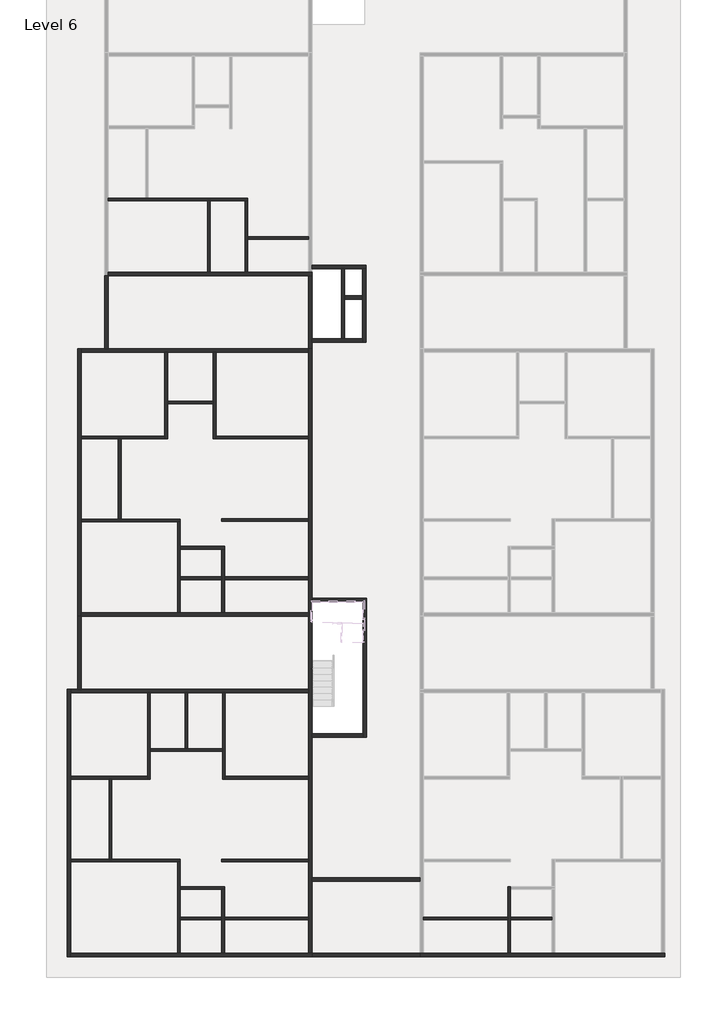
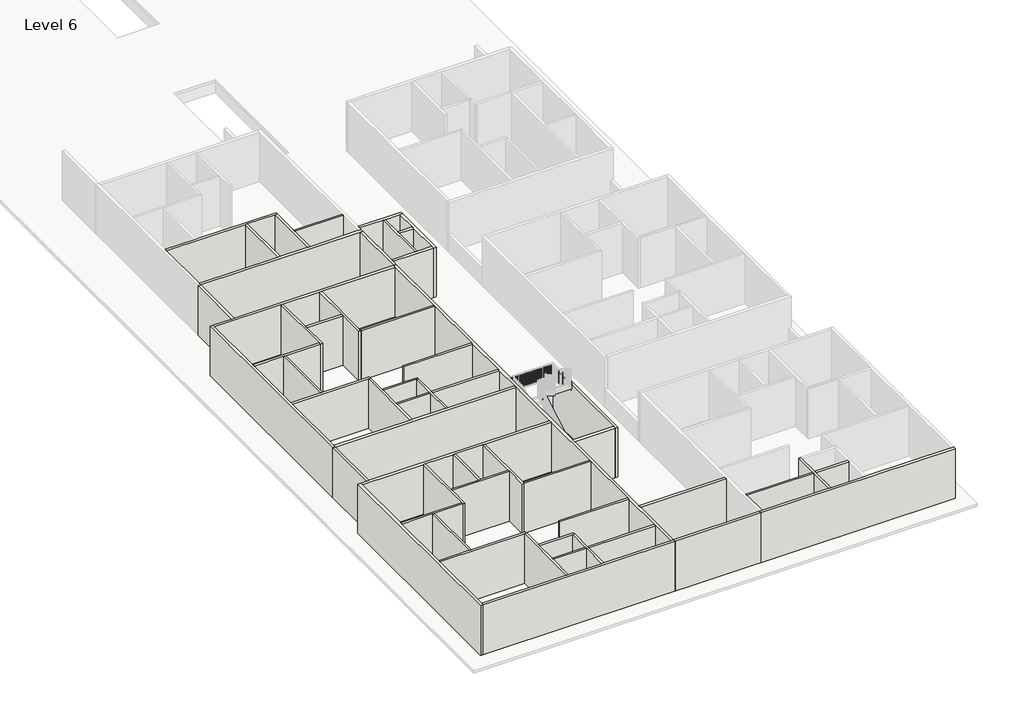
# One storey, part 1 of 8: 55 walls.
"""IFC4 building model written with IfcOpenShell, lengths in millimetres."""

from ifc_helpers import new_model, si_unit, frame, origin, place, context, project, spatial, polyline, outline, extrude, faceted_brep, element, save

model = new_model("IFC4")

# Units and contexts
model_context = context("Model", 3, world=origin())
ifc_project = project(units=[si_unit("LENGTHUNIT", "METRE", prefix="MILLI")], contexts=[model_context])

# Site, building, storey
site = spatial("IfcSite", under=ifc_project)
building = spatial("IfcBuilding", under=site)
storey = spatial("IfcBuildingStorey", under=building, Name="Level 6", Elevation=40474.6172466)

# Walls
placement = place(None, origin())
element("IfcWall", 1, ObjectType="4.5\"", at=placement, inside=storey, context=model_context, shape_type="Brep", body=[
    faceted_brep([(-12531.5544854, -1061.7344126, 40474.6172466), (-8188.1544854, -1061.7344126, 40474.6172466), (-8073.8544854, -1061.7344126, 40474.6172466), (-6549.8544854, -1061.7344126, 40474.6172466), (-6435.5544854, -1061.7344126, 40474.6172466), (-6435.5544854, -1061.7344126, 43522.6172466), (-6549.8544854, -1061.7344126, 43522.6172466), (-8073.8544854, -1061.7344126, 43522.6172466), (-8188.1544854, -1061.7344126, 43522.6172466), (-12531.5544854, -1061.7344126, 43522.6172466), (-12531.5544854, -947.4344126, 40474.6172466), (-12531.5544854, -947.4344126, 43522.6172466), (-10907.2415084, -947.4344126, 43522.6172466), (-10792.9415084, -947.4344126, 43522.6172466), (-6435.5544854, -947.4344126, 43522.6172466), (-6435.5544854, -947.4344126, 40474.6172466), (-10792.9415084, -947.4344126, 40474.6172466), (-10907.2415084, -947.4344126, 40474.6172466)], [[[0, 1, 2, 3, 4, 5, 6, 7, 8, 9]], [[10, 11, 12, 13, 14, 15, 16, 17]], [[4, 3, 2, 1, 0, 10, 17, 16, 15]], [[0, 9, 11, 10]], [[5, 4, 15, 14]], [[9, 8, 7, 6, 5, 14, 13, 12, 11]]]),
])
element("IfcWall", 2, ObjectType="4.5\"", at=placement, inside=storey, context=model_context, shape_type="Brep", body=[
    faceted_brep([(-6549.8544854, -1061.7344126, 40474.6172466), (-6549.8544854, -4185.9344126, 40474.6172466), (-6549.8544854, -4185.9344126, 43522.6172466), (-6549.8544854, -1061.7344126, 43522.6172466), (-6435.5544854, -1061.7344126, 40474.6172466), (-6435.5544854, -1061.7344126, 43522.6172466), (-6435.5544854, -2623.8344126, 43522.6172466), (-6435.5544854, -2738.1344126, 43522.6172466), (-6435.5544854, -4185.9344126, 43522.6172466), (-6435.5544854, -4185.9344126, 40474.6172466), (-6435.5544854, -2738.1344126, 40474.6172466), (-6435.5544854, -2623.8344126, 40474.6172466)], [[[0, 1, 2, 3]], [[4, 5, 6, 7, 8, 9, 10, 11]], [[1, 0, 4, 11, 10, 9]], [[0, 3, 5, 4]], [[2, 1, 9, 8]], [[3, 2, 8, 7, 6, 5]]]),
])
element("IfcWall", 3, ObjectType="4.5\"", at=placement, inside=storey, context=model_context, shape_type="SweptSolid", body=[
    extrude(outline(polyline([(-8188.1544854, -4185.9344126), (-8188.1544854, -1061.7344126), (-8073.8544854, -1061.7344126), (-8073.8544854, -4185.9344126), (-8188.1544854, -4185.9344126)])), frame((0.0, 0.0, 40474.6172466), z_axis=(0.0, 0.0, 1.0), x_axis=(1.0, 0.0, 0.0)), (0.0, 0.0, 1.0), 3048.0),
])
element("IfcWall", 4, ObjectType="4.5\"", at=placement, inside=storey, context=model_context, shape_type="SweptSolid", body=[
    extrude(outline(polyline([(-6435.5544854, -2623.8344126), (-3769.8415084, -2623.8344126), (-3769.8415084, -2738.1344126), (-6435.5544854, -2738.1344126), (-6435.5544854, -2623.8344126)])), frame((0.0, 0.0, 40474.6172466), z_axis=(0.0, 0.0, 1.0), x_axis=(1.0, 0.0, 0.0)), (0.0, 0.0, 1.0), 3048.0),
])
element("IfcWall", 5, ObjectType="4.5\"", at=placement, inside=storey, context=model_context, shape_type="Brep", body=[
    faceted_brep([(-10061.4044854, -7691.1344126, 40474.6172466), (-10061.4044854, -11348.7344126, 40474.6172466), (-10061.4044854, -11463.0344126, 40474.6172466), (-10061.4044854, -11463.0344126, 43522.6172466), (-10061.4044854, -11348.7344126, 43522.6172466), (-10061.4044854, -7691.1344126, 43522.6172466), (-9947.1044854, -7691.1344126, 40474.6172466), (-9947.1044854, -7691.1344126, 43522.6172466), (-9947.1044854, -9824.7344126, 43522.6172466), (-9947.1044854, -9939.0344126, 43522.6172466), (-9947.1044854, -11463.0344126, 43522.6172466), (-9947.1044854, -11463.0344126, 40474.6172466), (-9947.1044854, -9939.0344126, 40474.6172466), (-9947.1044854, -9824.7344126, 40474.6172466)], [[[0, 1, 2, 3, 4, 5]], [[6, 7, 8, 9, 10, 11, 12, 13]], [[2, 1, 0, 6, 13, 12, 11]], [[0, 5, 7, 6]], [[3, 2, 11, 10]], [[5, 4, 3, 10, 9, 8, 7]]]),
])
element("IfcWall", 6, ObjectType="4.5\"", at=placement, inside=storey, context=model_context, shape_type="Brep", body=[
    faceted_brep([(-10061.4044854, -11348.7344126, 40474.6172466), (-13719.0044854, -11348.7344126, 40474.6172466), (-13719.0044854, -11348.7344126, 43522.6172466), (-10061.4044854, -11348.7344126, 43522.6172466), (-10061.4044854, -11463.0344126, 40474.6172466), (-10061.4044854, -11463.0344126, 43522.6172466), (-11980.3915084, -11463.0344126, 43522.6172466), (-12094.6915084, -11463.0344126, 43522.6172466), (-13719.0044854, -11463.0344126, 43522.6172466), (-13719.0044854, -11463.0344126, 40474.6172466), (-12094.6915084, -11463.0344126, 40474.6172466), (-11980.3915084, -11463.0344126, 40474.6172466)], [[[0, 1, 2, 3]], [[4, 5, 6, 7, 8, 9, 10, 11]], [[1, 0, 4, 11, 10, 9]], [[0, 3, 5, 4]], [[2, 1, 9, 8]], [[3, 2, 8, 7, 6, 5]]]),
])
element("IfcWall", 7, ObjectType="4.5\"", at=placement, inside=storey, context=model_context, shape_type="SweptSolid", body=[
    extrude(outline(polyline([(-12094.6915084, -14968.2344126), (-12094.6915084, -11463.0344126), (-11980.3915084, -11463.0344126), (-11980.3915084, -14968.2344126), (-12094.6915084, -14968.2344126)])), frame((0.0, 0.0, 40474.6172466), z_axis=(0.0, 0.0, 1.0), x_axis=(1.0, 0.0, 0.0)), (0.0, 0.0, 1.0), 3048.0),
])
element("IfcWall", 8, ObjectType="4.5\"", at=placement, inside=storey, context=model_context, shape_type="Brep", body=[
    faceted_brep([(-13719.0044854, -15095.2344126, 40474.6172466), (-9510.2415084, -15095.2344126, 40474.6172466), (-9395.9415084, -15095.2344126, 40474.6172466), (-9395.9415084, -15095.2344126, 43522.6172466), (-9510.2415084, -15095.2344126, 43522.6172466), (-13719.0044854, -15095.2344126, 43522.6172466), (-13719.0044854, -14980.9344126, 40474.6172466), (-13719.0044854, -14980.9344126, 43522.6172466), (-9395.9415084, -14980.9344126, 43522.6172466), (-9395.9415084, -14980.9344126, 40474.6172466)], [[[0, 1, 2, 3, 4, 5]], [[6, 7, 8, 9]], [[2, 1, 0, 6, 9]], [[0, 5, 7, 6]], [[3, 2, 9, 8]], [[5, 4, 3, 8, 7]]]),
])
element("IfcWall", 9, ObjectType="4.5\"", at=placement, inside=storey, context=model_context, shape_type="Brep", body=[
    faceted_brep([(-9510.2415084, -15095.2344126, 40474.6172466), (-9510.2415084, -19070.3344126, 40474.6172466), (-9510.2415084, -19070.3344126, 43522.6172466), (-9510.2415084, -15095.2344126, 43522.6172466), (-9395.9415084, -15095.2344126, 40474.6172466), (-9395.9415084, -15095.2344126, 43522.6172466), (-9395.9415084, -16174.7344126, 43522.6172466), (-9395.9415084, -16289.0344126, 43522.6172466), (-9395.9415084, -17508.2344126, 43522.6172466), (-9395.9415084, -17622.5344126, 43522.6172466), (-9395.9415084, -19070.3344126, 43522.6172466), (-9395.9415084, -19070.3344126, 40474.6172466), (-9395.9415084, -17622.5344126, 40474.6172466), (-9395.9415084, -17508.2344126, 40474.6172466), (-9395.9415084, -16289.0344126, 40474.6172466), (-9395.9415084, -16174.7344126, 40474.6172466)], [[[0, 1, 2, 3]], [[4, 5, 6, 7, 8, 9, 10, 11, 12, 13, 14, 15]], [[1, 0, 4, 15, 14, 13, 12, 11]], [[0, 3, 5, 4]], [[2, 1, 11, 10]], [[3, 2, 10, 9, 8, 7, 6, 5]]]),
])
element("IfcWall", 10, ObjectType="4.5\"", at=placement, inside=storey, context=model_context, shape_type="Brep", body=[
    faceted_brep([(-9395.9415084, -16289.0344126, 40474.6172466), (-7567.1415084, -16289.0344126, 40474.6172466), (-7452.8415084, -16289.0344126, 40474.6172466), (-7452.8415084, -16289.0344126, 43522.6172466), (-7567.1415084, -16289.0344126, 43522.6172466), (-9395.9415084, -16289.0344126, 43522.6172466), (-9395.9415084, -16174.7344126, 40474.6172466), (-9395.9415084, -16174.7344126, 43522.6172466), (-7452.8415084, -16174.7344126, 43522.6172466), (-7452.8415084, -16174.7344126, 40474.6172466)], [[[0, 1, 2, 3, 4, 5]], [[6, 7, 8, 9]], [[2, 1, 0, 6, 9]], [[0, 5, 7, 6]], [[3, 2, 9, 8]], [[5, 4, 3, 8, 7]]]),
])
element("IfcWall", 11, ObjectType="4.5\"", at=placement, inside=storey, context=model_context, shape_type="Brep", body=[
    faceted_brep([(-7567.1415084, -16289.0344126, 40474.6172466), (-7567.1415084, -17508.2344126, 40474.6172466), (-7567.1415084, -17622.5344126, 40474.6172466), (-7567.1415084, -19070.3344126, 40474.6172466), (-7567.1415084, -19070.3344126, 43522.6172466), (-7567.1415084, -17622.5344126, 43522.6172466), (-7567.1415084, -17508.2344126, 43522.6172466), (-7567.1415084, -16289.0344126, 43522.6172466), (-7452.8415084, -16289.0344126, 40474.6172466), (-7452.8415084, -16289.0344126, 43522.6172466), (-7452.8415084, -17508.2344126, 43522.6172466), (-7452.8415084, -17622.5344126, 43522.6172466), (-7452.8415084, -19070.3344126, 43522.6172466), (-7452.8415084, -19070.3344126, 40474.6172466), (-7452.8415084, -17622.5344126, 40474.6172466), (-7452.8415084, -17508.2344126, 40474.6172466)], [[[0, 1, 2, 3, 4, 5, 6, 7]], [[8, 9, 10, 11, 12, 13, 14, 15]], [[3, 2, 1, 0, 8, 15, 14, 13]], [[0, 7, 9, 8]], [[4, 3, 13, 12]], [[7, 6, 5, 4, 12, 11, 10, 9]]]),
])
element("IfcWall", 12, ObjectType="4.5\"", at=placement, inside=storey, context=model_context, shape_type="SweptSolid", body=[
    extrude(outline(polyline([(-7567.1415084, -17622.5344126), (-9395.9415084, -17622.5344126), (-9395.9415084, -17508.2344126), (-7567.1415084, -17508.2344126), (-7567.1415084, -17622.5344126)])), frame((0.0, 0.0, 40474.6172466), z_axis=(0.0, 0.0, 1.0), x_axis=(1.0, 0.0, 0.0)), (0.0, 0.0, 1.0), 3048.0),
])
element("IfcWall", 13, ObjectType="4.5\"", at=placement, inside=storey, context=model_context, shape_type="SweptSolid", body=[
    extrude(outline(polyline([(-3769.8415084, -17622.5344126), (-7452.8415084, -17622.5344126), (-7452.8415084, -17508.2344126), (-3769.8415084, -17508.2344126), (-3769.8415084, -17622.5344126)])), frame((0.0, 0.0, 40474.6172466), z_axis=(0.0, 0.0, 1.0), x_axis=(1.0, 0.0, 0.0)), (0.0, 0.0, 1.0), 3048.0),
])
element("IfcWall", 14, ObjectType="4.5\"", at=placement, inside=storey, context=model_context, shape_type="SweptSolid", body=[
    extrude(outline(polyline([(-7567.1415084, -14968.2344126), (-3769.8415084, -14968.2344126), (-3769.8415084, -15082.5344126), (-7567.1415084, -15082.5344126), (-7567.1415084, -14968.2344126)])), frame((0.0, 0.0, 40474.6172466), z_axis=(0.0, 0.0, 1.0), x_axis=(1.0, 0.0, 0.0)), (0.0, 0.0, 1.0), 3048.0),
])
element("IfcWall", 15, ObjectType="4.5\"", at=placement, inside=storey, context=model_context, shape_type="SweptSolid", body=[
    extrude(outline(polyline([(-7940.5044854, -9939.0344126), (-9947.1044854, -9939.0344126), (-9947.1044854, -9824.7344126), (-7940.5044854, -9824.7344126), (-7940.5044854, -9939.0344126)])), frame((0.0, 0.0, 40474.6172466), z_axis=(0.0, 0.0, 1.0), x_axis=(1.0, 0.0, 0.0)), (0.0, 0.0, 1.0), 3048.0),
])
element("IfcWall", 16, ObjectType="4.5\"", at=placement, inside=storey, context=model_context, shape_type="Brep", body=[
    faceted_brep([(-7940.5044854, -7691.1344126, 40474.6172466), (-7940.5044854, -9824.7344126, 40474.6172466), (-7940.5044854, -9939.0344126, 40474.6172466), (-7940.5044854, -11463.0344126, 40474.6172466), (-7940.5044854, -11463.0344126, 43522.6172466), (-7940.5044854, -9939.0344126, 43522.6172466), (-7940.5044854, -9824.7344126, 43522.6172466), (-7940.5044854, -7691.1344126, 43522.6172466), (-7826.2044854, -7691.1344126, 40474.6172466), (-7826.2044854, -7691.1344126, 43522.6172466), (-7826.2044854, -11348.7344126, 43522.6172466), (-7826.2044854, -11463.0344126, 43522.6172466), (-7826.2044854, -11463.0344126, 40474.6172466), (-7826.2044854, -11348.7344126, 40474.6172466)], [[[0, 1, 2, 3, 4, 5, 6, 7]], [[8, 9, 10, 11, 12, 13]], [[3, 2, 1, 0, 8, 13, 12]], [[0, 7, 9, 8]], [[4, 3, 12, 11]], [[7, 6, 5, 4, 11, 10, 9]]]),
])
element("IfcWall", 17, ObjectType="4.5\"", at=placement, inside=storey, context=model_context, shape_type="SweptSolid", body=[
    extrude(outline(polyline([(-3769.8415084, -11463.0344126), (-7826.2044854, -11463.0344126), (-7826.2044854, -11348.7344126), (-3769.8415084, -11348.7344126), (-3769.8415084, -11463.0344126)])), frame((0.0, 0.0, 40474.6172466), z_axis=(0.0, 0.0, 1.0), x_axis=(1.0, 0.0, 0.0)), (0.0, 0.0, 1.0), 3048.0),
])
element("IfcWall", 18, ObjectType="4.5\"", at=placement, inside=storey, context=model_context, shape_type="Brep", body=[
    faceted_brep([(-10818.3415084, -22575.5344126, 40474.6172466), (-10818.3415084, -26233.1344126, 40474.6172466), (-10818.3415084, -26347.4344126, 40474.6172466), (-10818.3415084, -26347.4344126, 43522.6172466), (-10818.3415084, -26233.1344126, 43522.6172466), (-10818.3415084, -22575.5344126, 43522.6172466), (-10704.0415084, -22575.5344126, 40474.6172466), (-10704.0415084, -22575.5344126, 43522.6172466), (-10704.0415084, -25013.9344126, 43522.6172466), (-10704.0415084, -25128.2344126, 43522.6172466), (-10704.0415084, -26347.4344126, 43522.6172466), (-10704.0415084, -26347.4344126, 40474.6172466), (-10704.0415084, -25128.2344126, 40474.6172466), (-10704.0415084, -25013.9344126, 40474.6172466)], [[[0, 1, 2, 3, 4, 5]], [[6, 7, 8, 9, 10, 11, 12, 13]], [[2, 1, 0, 6, 13, 12, 11]], [[0, 5, 7, 6]], [[3, 2, 11, 10]], [[5, 4, 3, 10, 9, 8, 7]]]),
])
element("IfcWall", 19, ObjectType="4.5\"", at=placement, inside=storey, context=model_context, shape_type="Brep", body=[
    faceted_brep([(-10818.3415084, -26233.1344126, 40474.6172466), (-14171.1415084, -26233.1344126, 40474.6172466), (-14171.1415084, -26233.1344126, 43522.6172466), (-10818.3415084, -26233.1344126, 43522.6172466), (-10818.3415084, -26347.4344126, 40474.6172466), (-10818.3415084, -26347.4344126, 43522.6172466), (-12380.4415084, -26347.4344126, 43522.6172466), (-12494.7415084, -26347.4344126, 43522.6172466), (-14171.1415084, -26347.4344126, 43522.6172466), (-14171.1415084, -26347.4344126, 40474.6172466), (-12494.7415084, -26347.4344126, 40474.6172466), (-12380.4415084, -26347.4344126, 40474.6172466)], [[[0, 1, 2, 3]], [[4, 5, 6, 7, 8, 9, 10, 11]], [[1, 0, 4, 11, 10, 9]], [[0, 3, 5, 4]], [[2, 1, 9, 8]], [[3, 2, 8, 7, 6, 5]]]),
])
element("IfcWall", 20, ObjectType="4.5\"", at=placement, inside=storey, context=model_context, shape_type="SweptSolid", body=[
    extrude(outline(polyline([(-9180.0415084, -25013.9344126), (-9180.0415084, -22575.5344126), (-9065.7415084, -22575.5344126), (-9065.7415084, -25013.9344126), (-9180.0415084, -25013.9344126)])), frame((0.0, 0.0, 40474.6172466), z_axis=(0.0, 0.0, 1.0), x_axis=(1.0, 0.0, 0.0)), (0.0, 0.0, 1.0), 3048.0),
])
element("IfcWall", 21, ObjectType="4.5\"", at=placement, inside=storey, context=model_context, shape_type="Brep", body=[
    faceted_brep([(-10704.0415084, -25128.2344126, 40474.6172466), (-7541.7415084, -25128.2344126, 40474.6172466), (-7541.7415084, -25128.2344126, 43522.6172466), (-10704.0415084, -25128.2344126, 43522.6172466), (-10704.0415084, -25013.9344126, 40474.6172466), (-10704.0415084, -25013.9344126, 43522.6172466), (-9180.0415084, -25013.9344126, 43522.6172466), (-9065.7415084, -25013.9344126, 43522.6172466), (-7541.7415084, -25013.9344126, 43522.6172466), (-7541.7415084, -25013.9344126, 40474.6172466), (-9065.7415084, -25013.9344126, 40474.6172466), (-9180.0415084, -25013.9344126, 40474.6172466)], [[[0, 1, 2, 3]], [[4, 5, 6, 7, 8, 9, 10, 11]], [[1, 0, 4, 11, 10, 9]], [[0, 3, 5, 4]], [[2, 1, 9, 8]], [[3, 2, 8, 7, 6, 5]]]),
])
element("IfcWall", 22, ObjectType="4.5\"", at=placement, inside=storey, context=model_context, shape_type="Brep", body=[
    faceted_brep([(-7541.7415084, -22575.5344126, 40474.6172466), (-7541.7415084, -25013.9344126, 40474.6172466), (-7541.7415084, -25128.2344126, 40474.6172466), (-7541.7415084, -26347.4344126, 40474.6172466), (-7541.7415084, -26347.4344126, 43522.6172466), (-7541.7415084, -25128.2344126, 43522.6172466), (-7541.7415084, -25013.9344126, 43522.6172466), (-7541.7415084, -22575.5344126, 43522.6172466), (-7427.4415084, -22575.5344126, 40474.6172466), (-7427.4415084, -22575.5344126, 43522.6172466), (-7427.4415084, -26233.1344126, 43522.6172466), (-7427.4415084, -26347.4344126, 43522.6172466), (-7427.4415084, -26347.4344126, 40474.6172466), (-7427.4415084, -26233.1344126, 40474.6172466)], [[[0, 1, 2, 3, 4, 5, 6, 7]], [[8, 9, 10, 11, 12, 13]], [[3, 2, 1, 0, 8, 13, 12]], [[0, 7, 9, 8]], [[4, 3, 12, 11]], [[7, 6, 5, 4, 11, 10, 9]]]),
])
element("IfcWall", 23, ObjectType="4.5\"", at=placement, inside=storey, context=model_context, shape_type="SweptSolid", body=[
    extrude(outline(polyline([(-3769.8415084, -26347.4344126), (-7427.4415084, -26347.4344126), (-7427.4415084, -26233.1344126), (-3769.8415084, -26233.1344126), (-3769.8415084, -26347.4344126)])), frame((0.0, 0.0, 40474.6172466), z_axis=(0.0, 0.0, 1.0), x_axis=(1.0, 0.0, 0.0)), (0.0, 0.0, 1.0), 3048.0),
])
element("IfcWall", 24, ObjectType="4.5\"", at=placement, inside=storey, context=model_context, shape_type="SweptSolid", body=[
    extrude(outline(polyline([(-12494.7415084, -29852.6344126), (-12494.7415084, -26347.4344126), (-12380.4415084, -26347.4344126), (-12380.4415084, -29852.6344126), (-12494.7415084, -29852.6344126)])), frame((0.0, 0.0, 40474.6172466), z_axis=(0.0, 0.0, 1.0), x_axis=(1.0, 0.0, 0.0)), (0.0, 0.0, 1.0), 3048.0),
])
element("IfcWall", 25, ObjectType="4.5\"", at=placement, inside=storey, context=model_context, shape_type="Brep", body=[
    faceted_brep([(-14171.1415084, -29966.9344126, 40474.6172466), (-9510.2415084, -29966.9344126, 40474.6172466), (-9395.9415084, -29966.9344126, 40474.6172466), (-9395.9415084, -29966.9344126, 43522.6172466), (-9510.2415084, -29966.9344126, 43522.6172466), (-14171.1415084, -29966.9344126, 43522.6172466), (-14171.1415084, -29852.6344126, 40474.6172466), (-14171.1415084, -29852.6344126, 43522.6172466), (-12494.7415084, -29852.6344126, 43522.6172466), (-12380.4415084, -29852.6344126, 43522.6172466), (-9395.9415084, -29852.6344126, 43522.6172466), (-9395.9415084, -29852.6344126, 40474.6172466), (-12380.4415084, -29852.6344126, 40474.6172466), (-12494.7415084, -29852.6344126, 40474.6172466)], [[[0, 1, 2, 3, 4, 5]], [[6, 7, 8, 9, 10, 11, 12, 13]], [[2, 1, 0, 6, 13, 12, 11]], [[0, 5, 7, 6]], [[3, 2, 11, 10]], [[5, 4, 3, 10, 9, 8, 7]]]),
])
element("IfcWall", 26, ObjectType="4.5\"", at=placement, inside=storey, context=model_context, shape_type="Brep", body=[
    faceted_brep([(-9510.2415084, -29966.9344126, 40474.6172466), (-9510.2415084, -33954.7344126, 40474.6172466), (-9510.2415084, -33954.7344126, 43522.6172466), (-9510.2415084, -29966.9344126, 43522.6172466), (-9395.9415084, -29966.9344126, 40474.6172466), (-9395.9415084, -29966.9344126, 43522.6172466), (-9395.9415084, -31059.1344126, 43522.6172466), (-9395.9415084, -31173.4344126, 43522.6172466), (-9395.9415084, -32392.6344126, 43522.6172466), (-9395.9415084, -32506.9344126, 43522.6172466), (-9395.9415084, -33954.7344126, 43522.6172466), (-9395.9415084, -33954.7344126, 40474.6172466), (-9395.9415084, -32506.9344126, 40474.6172466), (-9395.9415084, -32392.6344126, 40474.6172466), (-9395.9415084, -31173.4344126, 40474.6172466), (-9395.9415084, -31059.1344126, 40474.6172466)], [[[0, 1, 2, 3]], [[4, 5, 6, 7, 8, 9, 10, 11, 12, 13, 14, 15]], [[1, 0, 4, 15, 14, 13, 12, 11]], [[0, 3, 5, 4]], [[2, 1, 11, 10]], [[3, 2, 10, 9, 8, 7, 6, 5]]]),
])
element("IfcWall", 27, ObjectType="4.5\"", at=placement, inside=storey, context=model_context, shape_type="Brep", body=[
    faceted_brep([(-9395.9415084, -31173.4344126, 40474.6172466), (-7567.1415084, -31173.4344126, 40474.6172466), (-7452.8415084, -31173.4344126, 40474.6172466), (-7452.8415084, -31173.4344126, 43522.6172466), (-7567.1415084, -31173.4344126, 43522.6172466), (-9395.9415084, -31173.4344126, 43522.6172466), (-9395.9415084, -31059.1344126, 40474.6172466), (-9395.9415084, -31059.1344126, 43522.6172466), (-7452.8415084, -31059.1344126, 43522.6172466), (-7452.8415084, -31059.1344126, 40474.6172466)], [[[0, 1, 2, 3, 4, 5]], [[6, 7, 8, 9]], [[2, 1, 0, 6, 9]], [[0, 5, 7, 6]], [[3, 2, 9, 8]], [[5, 4, 3, 8, 7]]]),
])
element("IfcWall", 28, ObjectType="4.5\"", at=placement, inside=storey, context=model_context, shape_type="Brep", body=[
    faceted_brep([(-7567.1415084, -31173.4344126, 40474.6172466), (-7567.1415084, -32392.6344126, 40474.6172466), (-7567.1415084, -32506.9344126, 40474.6172466), (-7567.1415084, -33954.7344126, 40474.6172466), (-7567.1415084, -33954.7344126, 43522.6172466), (-7567.1415084, -32506.9344126, 43522.6172466), (-7567.1415084, -32392.6344126, 43522.6172466), (-7567.1415084, -31173.4344126, 43522.6172466), (-7452.8415084, -31173.4344126, 40474.6172466), (-7452.8415084, -31173.4344126, 43522.6172466), (-7452.8415084, -32392.6344126, 43522.6172466), (-7452.8415084, -32506.9344126, 43522.6172466), (-7452.8415084, -33954.7344126, 43522.6172466), (-7452.8415084, -33954.7344126, 40474.6172466), (-7452.8415084, -32506.9344126, 40474.6172466), (-7452.8415084, -32392.6344126, 40474.6172466)], [[[0, 1, 2, 3, 4, 5, 6, 7]], [[8, 9, 10, 11, 12, 13, 14, 15]], [[3, 2, 1, 0, 8, 15, 14, 13]], [[0, 7, 9, 8]], [[4, 3, 13, 12]], [[7, 6, 5, 4, 12, 11, 10, 9]]]),
])
element("IfcWall", 29, ObjectType="4.5\"", at=placement, inside=storey, context=model_context, shape_type="SweptSolid", body=[
    extrude(outline(polyline([(-3769.8415084, -32392.6344126), (-3769.8415084, -32506.9344126), (-7452.8415084, -32506.9344126), (-7452.8415084, -32392.6344126), (-3769.8415084, -32392.6344126)])), frame((0.0, 0.0, 40474.6172466), z_axis=(0.0, 0.0, 1.0), x_axis=(1.0, 0.0, 0.0)), (0.0, 0.0, 1.0), 3048.0),
    extrude(outline(polyline([(-9395.9415084, -32506.9344126), (-9395.9415084, -32392.6344126), (-7567.1415084, -32392.6344126), (-7567.1415084, -32506.9344126), (-9395.9415084, -32506.9344126)])), frame((0.0, 0.0, 40474.6172466), z_axis=(0.0, 0.0, 1.0), x_axis=(1.0, 0.0, 0.0)), (0.0, 0.0, 1.0), 3048.0),
])
element("IfcWall", 30, ObjectType="4.5\"", at=placement, inside=storey, context=model_context, shape_type="SweptSolid", body=[
    extrude(outline(polyline([(-7567.1415084, -29852.6344126), (-3769.8415084, -29852.6344126), (-3769.8415084, -29966.9344126), (-7567.1415084, -29966.9344126), (-7567.1415084, -29852.6344126)])), frame((0.0, 0.0, 40474.6172466), z_axis=(0.0, 0.0, 1.0), x_axis=(1.0, 0.0, 0.0)), (0.0, 0.0, 1.0), 3048.0),
])
element("IfcWall", 31, ObjectType="4.5\"", at=placement, inside=storey, context=model_context, shape_type="SweptSolid", body=[
    extrude(outline(polyline([(4942.3584916, -32506.9344126), (1259.3584916, -32506.9344126), (1259.3584916, -32392.6344126), (4942.3584916, -32392.6344126), (4942.3584916, -32506.9344126)])), frame((0.0, 0.0, 40474.6172466), z_axis=(0.0, 0.0, 1.0), x_axis=(1.0, 0.0, 0.0)), (0.0, 0.0, 1.0), 3048.0),
])
element("IfcWall", 32, ObjectType="4.5\"", at=placement, inside=storey, context=model_context, shape_type="Brep", body=[
    faceted_brep([(4942.3584916, -31059.1344126, 40474.6172466), (4942.3584916, -32392.6344126, 40474.6172466), (4942.3584916, -32506.9344126, 40474.6172466), (4942.3584916, -33954.7344126, 40474.6172466), (4942.3584916, -33954.7344126, 43522.6172466), (4942.3584916, -32506.9344126, 43522.6172466), (4942.3584916, -32392.6344126, 43522.6172466), (4942.3584916, -31059.1344126, 43522.6172466), (5056.6584916, -31059.1344126, 40474.6172466), (5056.6584916, -31059.1344126, 43522.6172466), (5056.6584916, -31173.4344126, 43522.6172466), (5056.6584916, -32392.6344126, 43522.6172466), (5056.6584916, -32506.9344126, 43522.6172466), (5056.6584916, -33954.7344126, 43522.6172466), (5056.6584916, -33954.7344126, 40474.6172466), (5056.6584916, -32506.9344126, 40474.6172466), (5056.6584916, -32392.6344126, 40474.6172466), (5056.6584916, -31173.4344126, 40474.6172466)], [[[0, 1, 2, 3, 4, 5, 6, 7]], [[8, 9, 10, 11, 12, 13, 14, 15, 16, 17]], [[3, 2, 1, 0, 8, 17, 16, 15, 14]], [[4, 3, 14, 13]], [[0, 7, 9, 8]], [[7, 6, 5, 4, 13, 12, 11, 10, 9]]]),
])
element("IfcWall", 33, ObjectType="4.5\"", at=placement, inside=storey, context=model_context, shape_type="SweptSolid", body=[
    extrude(outline(polyline([(6885.4584916, -32506.9344126), (5056.6584916, -32506.9344126), (5056.6584916, -32392.6344126), (6885.4584916, -32392.6344126), (6885.4584916, -32506.9344126)])), frame((0.0, 0.0, 40474.6172466), z_axis=(0.0, 0.0, 1.0), x_axis=(1.0, 0.0, 0.0)), (0.0, 0.0, 1.0), 3048.0),
])
element("IfcWall", 34, ObjectType="4.5\"", at=placement, inside=storey, context=model_context, shape_type="Brep", body=[
    faceted_brep([(-2207.6738684, -7082.6751812, 40474.6172466), (-2207.6738684, -5366.3479894, 40474.6172466), (-2207.6738684, -5213.9479894, 40474.6172466), (-2207.6738684, -4034.6751812, 40474.6172466), (-2207.6738684, -4034.6751812, 43522.6172466), (-2207.6738684, -5213.9479894, 43522.6172466), (-2207.6738684, -5366.3479894, 43522.6172466), (-2207.6738684, -7082.6751812, 43522.6172466), (-2321.9738684, -7082.6751812, 40474.6172466), (-2321.9738684, -7082.6751812, 43522.6172466), (-2321.9738684, -4034.6751812, 43522.6172466), (-2321.9738684, -4034.6751812, 40474.6172466)], [[[0, 1, 2, 3, 4, 5, 6, 7]], [[8, 9, 10, 11]], [[3, 2, 1, 0, 8, 11]], [[7, 6, 5, 4, 10, 9]], [[4, 3, 11, 10]], [[0, 7, 9, 8]]]),
])
element("IfcWall", 35, ObjectType="6\"", at=placement, inside=storey, context=model_context, shape_type="Brep", body=[
    faceted_brep([(-12531.5544854, -4338.3344126, 40474.6172466), (-3769.8415084, -4338.3344126, 40474.6172466), (-3617.4415084, -4338.3344126, 40474.6172466), (-3617.4415084, -4338.3344126, 43522.6172466), (-3769.8415084, -4338.3344126, 43522.6172466), (-12531.5544854, -4338.3344126, 43522.6172466), (-12531.5544854, -4185.9344126, 40474.6172466), (-12531.5544854, -4185.9344126, 43522.6172466), (-8188.1544854, -4185.9344126, 43522.6172466), (-8073.8544854, -4185.9344126, 43522.6172466), (-6549.8544854, -4185.9344126, 43522.6172466), (-6435.5544854, -4185.9344126, 43522.6172466), (-3769.8415084, -4185.9344126, 43522.6172466), (-3617.4415084, -4185.9344126, 43522.6172466), (-3617.4415084, -4185.9344126, 40474.6172466), (-3769.8415084, -4185.9344126, 40474.6172466), (-6435.5544854, -4185.9344126, 40474.6172466), (-6549.8544854, -4185.9344126, 40474.6172466), (-8073.8544854, -4185.9344126, 40474.6172466), (-8188.1544854, -4185.9344126, 40474.6172466)], [[[0, 1, 2, 3, 4, 5]], [[6, 7, 8, 9, 10, 11, 12, 13, 14, 15, 16, 17, 18, 19]], [[2, 1, 0, 6, 19, 18, 17, 16, 15, 14]], [[0, 5, 7, 6]], [[3, 2, 14, 13]], [[5, 4, 3, 13, 12, 11, 10, 9, 8, 7]]]),
])
element("IfcWall", 36, ObjectType="6\"", at=placement, inside=storey, context=model_context, shape_type="Brep", body=[
    faceted_brep([(-13871.4044854, -7538.7344126, 40474.6172466), (-13871.4044854, -19222.7344126, 40474.6172466), (-13871.4044854, -19222.7344126, 43522.6172466), (-13871.4044854, -7538.7344126, 43522.6172466), (-13719.0044854, -7538.7344126, 40474.6172466), (-13719.0044854, -7538.7344126, 43522.6172466), (-13719.0044854, -7691.1344126, 43522.6172466), (-13719.0044854, -11348.7344126, 43522.6172466), (-13719.0044854, -11463.0344126, 43522.6172466), (-13719.0044854, -14980.9344126, 43522.6172466), (-13719.0044854, -15095.2344126, 43522.6172466), (-13719.0044854, -19070.3344126, 43522.6172466), (-13719.0044854, -19222.7344126, 43522.6172466), (-13719.0044854, -19222.7344126, 40474.6172466), (-13719.0044854, -19070.3344126, 40474.6172466), (-13719.0044854, -15095.2344126, 40474.6172466), (-13719.0044854, -14980.9344126, 40474.6172466), (-13719.0044854, -11463.0344126, 40474.6172466), (-13719.0044854, -11348.7344126, 40474.6172466), (-13719.0044854, -7691.1344126, 40474.6172466)], [[[0, 1, 2, 3]], [[4, 5, 6, 7, 8, 9, 10, 11, 12, 13, 14, 15, 16, 17, 18, 19]], [[1, 0, 4, 19, 18, 17, 16, 15, 14, 13]], [[2, 1, 13, 12]], [[0, 3, 5, 4]], [[3, 2, 12, 11, 10, 9, 8, 7, 6, 5]]]),
])
element("IfcWall", 37, ObjectType="6\"", at=placement, inside=storey, context=model_context, shape_type="Brep", body=[
    faceted_brep([(-13719.0044854, -19222.7344126, 40474.6172466), (-3769.8415084, -19222.7344126, 40474.6172466), (-3769.8415084, -19222.7344126, 43522.6172466), (-13719.0044854, -19222.7344126, 43522.6172466), (-13719.0044854, -19070.3344126, 40474.6172466), (-13719.0044854, -19070.3344126, 43522.6172466), (-9510.2415084, -19070.3344126, 43522.6172466), (-9395.9415084, -19070.3344126, 43522.6172466), (-7567.1415084, -19070.3344126, 43522.6172466), (-7452.8415084, -19070.3344126, 43522.6172466), (-3769.8415084, -19070.3344126, 43522.6172466), (-3769.8415084, -19070.3344126, 40474.6172466), (-7452.8415084, -19070.3344126, 40474.6172466), (-7567.1415084, -19070.3344126, 40474.6172466), (-9395.9415084, -19070.3344126, 40474.6172466), (-9510.2415084, -19070.3344126, 40474.6172466)], [[[0, 1, 2, 3]], [[4, 5, 6, 7, 8, 9, 10, 11, 12, 13, 14, 15]], [[1, 0, 4, 15, 14, 13, 12, 11]], [[0, 3, 5, 4]], [[2, 1, 11, 10]], [[3, 2, 10, 9, 8, 7, 6, 5]]]),
])
element("IfcWall", 38, ObjectType="6\"", at=placement, inside=storey, context=model_context, shape_type="Brep", body=[
    faceted_brep([(-3617.4415084, -33954.7344126, 40474.6172466), (-3617.4415084, -30820.9325185, 40474.6172466), (-3617.4415084, -30668.5325185, 40474.6172466), (-3617.4415084, -24525.9851539, 40474.6172466), (-3617.4415084, -24373.5851539, 40474.6172466), (-3617.4415084, -18582.3851539, 40474.6172466), (-3617.4415084, -18429.9851539, 40474.6172466), (-3617.4415084, -7538.7344126, 40474.6172466), (-3617.4415084, -7538.7344126, 43522.6172466), (-3617.4415084, -18429.9851539, 43522.6172466), (-3617.4415084, -18582.3851539, 43522.6172466), (-3617.4415084, -24373.5851539, 43522.6172466), (-3617.4415084, -24525.9851539, 43522.6172466), (-3617.4415084, -30668.5325185, 43522.6172466), (-3617.4415084, -30820.9325185, 43522.6172466), (-3617.4415084, -33954.7344126, 43522.6172466), (-3769.8415084, -33954.7344126, 40474.6172466), (-3769.8415084, -33954.7344126, 43522.6172466), (-3769.8415084, -32506.9344126, 43522.6172466), (-3769.8415084, -32392.6344126, 43522.6172466), (-3769.8415084, -29966.9344126, 43522.6172466), (-3769.8415084, -29852.6344126, 43522.6172466), (-3769.8415084, -26347.4344126, 43522.6172466), (-3769.8415084, -26233.1344126, 43522.6172466), (-3769.8415084, -22575.5344126, 43522.6172466), (-3769.8415084, -22423.1344126, 43522.6172466), (-3769.8415084, -19222.7344126, 43522.6172466), (-3769.8415084, -19070.3344126, 43522.6172466), (-3769.8415084, -17622.5344126, 43522.6172466), (-3769.8415084, -17508.2344126, 43522.6172466), (-3769.8415084, -15082.5344126, 43522.6172466), (-3769.8415084, -14968.2344126, 43522.6172466), (-3769.8415084, -11463.0344126, 43522.6172466), (-3769.8415084, -11348.7344126, 43522.6172466), (-3769.8415084, -7691.1344126, 43522.6172466), (-3769.8415084, -7538.7344126, 43522.6172466), (-3769.8415084, -7538.7344126, 40474.6172466), (-3769.8415084, -7691.1344126, 40474.6172466), (-3769.8415084, -11348.7344126, 40474.6172466), (-3769.8415084, -11463.0344126, 40474.6172466), (-3769.8415084, -14968.2344126, 40474.6172466), (-3769.8415084, -15082.5344126, 40474.6172466), (-3769.8415084, -17508.2344126, 40474.6172466), (-3769.8415084, -17622.5344126, 40474.6172466), (-3769.8415084, -19070.3344126, 40474.6172466), (-3769.8415084, -19222.7344126, 40474.6172466), (-3769.8415084, -22423.1344126, 40474.6172466), (-3769.8415084, -22575.5344126, 40474.6172466), (-3769.8415084, -26233.1344126, 40474.6172466), (-3769.8415084, -26347.4344126, 40474.6172466), (-3769.8415084, -29852.6344126, 40474.6172466), (-3769.8415084, -29966.9344126, 40474.6172466), (-3769.8415084, -32392.6344126, 40474.6172466), (-3769.8415084, -32506.9344126, 40474.6172466)], [[[0, 1, 2, 3, 4, 5, 6, 7, 8, 9, 10, 11, 12, 13, 14, 15]], [[16, 17, 18, 19, 20, 21, 22, 23, 24, 25, 26, 27, 28, 29, 30, 31, 32, 33, 34, 35, 36, 37, 38, 39, 40, 41, 42, 43, 44, 45, 46, 47, 48, 49, 50, 51, 52, 53]], [[7, 6, 5, 4, 3, 2, 1, 0, 16, 53, 52, 51, 50, 49, 48, 47, 46, 45, 44, 43, 42, 41, 40, 39, 38, 37, 36]], [[8, 7, 36, 35]], [[0, 15, 17, 16]], [[15, 14, 13, 12, 11, 10, 9, 8, 35, 34, 33, 32, 31, 30, 29, 28, 27, 26, 25, 24, 23, 22, 21, 20, 19, 18, 17]]]),
])
element("IfcWall", 39, ObjectType="6\"", at=placement, inside=storey, context=model_context, shape_type="Brep", body=[
    faceted_brep([(-3769.8415084, -7538.7344126, 40474.6172466), (-12531.5544854, -7538.7344126, 40474.6172466), (-12683.9544854, -7538.7344126, 40474.6172466), (-13719.0044854, -7538.7344126, 40474.6172466), (-13719.0044854, -7538.7344126, 43522.6172466), (-12683.9544854, -7538.7344126, 43522.6172466), (-12531.5544854, -7538.7344126, 43522.6172466), (-3769.8415084, -7538.7344126, 43522.6172466), (-3769.8415084, -7691.1344126, 40474.6172466), (-3769.8415084, -7691.1344126, 43522.6172466), (-7826.2044854, -7691.1344126, 43522.6172466), (-7940.5044854, -7691.1344126, 43522.6172466), (-9947.1044854, -7691.1344126, 43522.6172466), (-10061.4044854, -7691.1344126, 43522.6172466), (-13719.0044854, -7691.1344126, 43522.6172466), (-13719.0044854, -7691.1344126, 40474.6172466), (-10061.4044854, -7691.1344126, 40474.6172466), (-9947.1044854, -7691.1344126, 40474.6172466), (-7940.5044854, -7691.1344126, 40474.6172466), (-7826.2044854, -7691.1344126, 40474.6172466)], [[[0, 1, 2, 3, 4, 5, 6, 7]], [[8, 9, 10, 11, 12, 13, 14, 15, 16, 17, 18, 19]], [[3, 2, 1, 0, 8, 19, 18, 17, 16, 15]], [[0, 7, 9, 8]], [[4, 3, 15, 14]], [[7, 6, 5, 4, 14, 13, 12, 11, 10, 9]]]),
])
element("IfcWall", 40, ObjectType="6\"", at=placement, inside=storey, context=model_context, shape_type="Brep", body=[
    faceted_brep([(-14323.5415084, -22423.1344126, 40474.6172466), (-14323.5415084, -34107.1344126, 40474.6172466), (-14323.5415084, -34107.1344126, 43522.6172466), (-14323.5415084, -22423.1344126, 43522.6172466), (-14171.1415084, -22423.1344126, 40474.6172466), (-14171.1415084, -22423.1344126, 43522.6172466), (-14171.1415084, -22575.5344126, 43522.6172466), (-14171.1415084, -26233.1344126, 43522.6172466), (-14171.1415084, -26347.4344126, 43522.6172466), (-14171.1415084, -29852.6344126, 43522.6172466), (-14171.1415084, -29966.9344126, 43522.6172466), (-14171.1415084, -33954.7344126, 43522.6172466), (-14171.1415084, -34107.1344126, 43522.6172466), (-14171.1415084, -34107.1344126, 40474.6172466), (-14171.1415084, -33954.7344126, 40474.6172466), (-14171.1415084, -29966.9344126, 40474.6172466), (-14171.1415084, -29852.6344126, 40474.6172466), (-14171.1415084, -26347.4344126, 40474.6172466), (-14171.1415084, -26233.1344126, 40474.6172466), (-14171.1415084, -22575.5344126, 40474.6172466)], [[[0, 1, 2, 3]], [[4, 5, 6, 7, 8, 9, 10, 11, 12, 13, 14, 15, 16, 17, 18, 19]], [[1, 0, 4, 19, 18, 17, 16, 15, 14, 13]], [[2, 1, 13, 12]], [[0, 3, 5, 4]], [[3, 2, 12, 11, 10, 9, 8, 7, 6, 5]]]),
])
element("IfcWall", 41, ObjectType="6\"", at=placement, inside=storey, context=model_context, shape_type="Brep", body=[
    faceted_brep([(-14171.1415084, -34107.1344126, 40474.6172466), (-3617.4415084, -34107.1344126, 40474.6172466), (-3617.4415084, -34107.1344126, 43522.6172466), (-14171.1415084, -34107.1344126, 43522.6172466), (-14171.1415084, -33954.7344126, 40474.6172466), (-14171.1415084, -33954.7344126, 43522.6172466), (-9510.2415084, -33954.7344126, 43522.6172466), (-9395.9415084, -33954.7344126, 43522.6172466), (-7567.1415084, -33954.7344126, 43522.6172466), (-7452.8415084, -33954.7344126, 43522.6172466), (-3769.8415084, -33954.7344126, 43522.6172466), (-3617.4415084, -33954.7344126, 43522.6172466), (-3617.4415084, -33954.7344126, 40474.6172466), (-3769.8415084, -33954.7344126, 40474.6172466), (-7452.8415084, -33954.7344126, 40474.6172466), (-7567.1415084, -33954.7344126, 40474.6172466), (-9395.9415084, -33954.7344126, 40474.6172466), (-9510.2415084, -33954.7344126, 40474.6172466)], [[[0, 1, 2, 3]], [[4, 5, 6, 7, 8, 9, 10, 11, 12, 13, 14, 15, 16, 17]], [[1, 0, 4, 17, 16, 15, 14, 13, 12]], [[0, 3, 5, 4]], [[2, 1, 12, 11]], [[3, 2, 11, 10, 9, 8, 7, 6, 5]]]),
])
element("IfcWall", 42, ObjectType="6\"", at=placement, inside=storey, context=model_context, shape_type="Brep", body=[
    faceted_brep([(-3769.8415084, -22423.1344126, 40474.6172466), (-13719.0044854, -22423.1344126, 40474.6172466), (-13871.4044854, -22423.1344126, 40474.6172466), (-14171.1415084, -22423.1344126, 40474.6172466), (-14171.1415084, -22423.1344126, 43522.6172466), (-13871.4044854, -22423.1344126, 43522.6172466), (-13719.0044854, -22423.1344126, 43522.6172466), (-3769.8415084, -22423.1344126, 43522.6172466), (-3769.8415084, -22575.5344126, 40474.6172466), (-3769.8415084, -22575.5344126, 43522.6172466), (-7427.4415084, -22575.5344126, 43522.6172466), (-7541.7415084, -22575.5344126, 43522.6172466), (-9065.7415084, -22575.5344126, 43522.6172466), (-9180.0415084, -22575.5344126, 43522.6172466), (-10704.0415084, -22575.5344126, 43522.6172466), (-10818.3415084, -22575.5344126, 43522.6172466), (-14171.1415084, -22575.5344126, 43522.6172466), (-14171.1415084, -22575.5344126, 40474.6172466), (-10818.3415084, -22575.5344126, 40474.6172466), (-10704.0415084, -22575.5344126, 40474.6172466), (-9180.0415084, -22575.5344126, 40474.6172466), (-9065.7415084, -22575.5344126, 40474.6172466), (-7541.7415084, -22575.5344126, 40474.6172466), (-7427.4415084, -22575.5344126, 40474.6172466)], [[[0, 1, 2, 3, 4, 5, 6, 7]], [[8, 9, 10, 11, 12, 13, 14, 15, 16, 17, 18, 19, 20, 21, 22, 23]], [[3, 2, 1, 0, 8, 23, 22, 21, 20, 19, 18, 17]], [[0, 7, 9, 8]], [[4, 3, 17, 16]], [[7, 6, 5, 4, 16, 15, 14, 13, 12, 11, 10, 9]]]),
])
element("IfcWall", 43, ObjectType="6\"", at=placement, inside=storey, context=model_context, shape_type="Brep", body=[
    faceted_brep([(1106.9584916, -34107.1344126, 40474.6172466), (11813.0584916, -34107.1344126, 40474.6172466), (11813.0584916, -34107.1344126, 43522.6172466), (1106.9584916, -34107.1344126, 43522.6172466), (1106.9584916, -33954.7344126, 40474.6172466), (1106.9584916, -33954.7344126, 43522.6172466), (1259.3584916, -33954.7344126, 43522.6172466), (4942.3584916, -33954.7344126, 43522.6172466), (5056.6584916, -33954.7344126, 43522.6172466), (6885.4584916, -33954.7344126, 43522.6172466), (6999.7584916, -33954.7344126, 43522.6172466), (11660.6584916, -33954.7344126, 43522.6172466), (11813.0584916, -33954.7344126, 43522.6172466), (11813.0584916, -33954.7344126, 40474.6172466), (11660.6584916, -33954.7344126, 40474.6172466), (6999.7584916, -33954.7344126, 40474.6172466), (6885.4584916, -33954.7344126, 40474.6172466), (5056.6584916, -33954.7344126, 40474.6172466), (4942.3584916, -33954.7344126, 40474.6172466), (1259.3584916, -33954.7344126, 40474.6172466)], [[[0, 1, 2, 3]], [[4, 5, 6, 7, 8, 9, 10, 11, 12, 13, 14, 15, 16, 17, 18, 19]], [[1, 0, 4, 19, 18, 17, 16, 15, 14, 13]], [[2, 1, 13, 12]], [[0, 3, 5, 4]], [[3, 2, 12, 11, 10, 9, 8, 7, 6, 5]]]),
])
element("IfcWall", 44, ObjectType="6\"", at=placement, inside=storey, context=model_context, shape_type="Brep", body=[
    faceted_brep([(-3617.4415084, -18582.3851539, 40474.6172466), (-1382.2415084, -18582.3851539, 40474.6172466), (-1229.8415084, -18582.3851539, 40474.6172466), (-1229.8415084, -18582.3851539, 43522.6172466), (-1382.2415084, -18582.3851539, 43522.6172466), (-3617.4415084, -18582.3851539, 43522.6172466), (-3617.4415084, -18429.9851539, 40474.6172466), (-3617.4415084, -18429.9851539, 43522.6172466), (-1229.8415084, -18429.9851539, 43522.6172466), (-1229.8415084, -18429.9851539, 40474.6172466)], [[[0, 1, 2, 3, 4, 5]], [[6, 7, 8, 9]], [[2, 1, 0, 6, 9]], [[5, 4, 3, 8, 7]], [[0, 5, 7, 6]], [[3, 2, 9, 8]]]),
])
element("IfcWall", 45, ObjectType="6\"", at=placement, inside=storey, context=model_context, shape_type="Brep", body=[
    faceted_brep([(-1382.2415084, -18582.3851539, 40474.6172466), (-1382.2415084, -24373.5851539, 40474.6172466), (-1382.2415084, -24525.9851539, 40474.6172466), (-1382.2415084, -24525.9851539, 43522.6172466), (-1382.2415084, -24373.5851539, 43522.6172466), (-1382.2415084, -18582.3851539, 43522.6172466), (-1229.8415084, -18582.3851539, 40474.6172466), (-1229.8415084, -18582.3851539, 43522.6172466), (-1229.8415084, -24525.9851539, 43522.6172466), (-1229.8415084, -24525.9851539, 40474.6172466)], [[[0, 1, 2, 3, 4, 5]], [[6, 7, 8, 9]], [[2, 1, 0, 6, 9]], [[5, 4, 3, 8, 7]], [[0, 5, 7, 6]], [[3, 2, 9, 8]]]),
])
element("IfcWall", 46, ObjectType="6\"", at=placement, inside=storey, context=model_context, shape_type="SweptSolid", body=[
    extrude(outline(polyline([(-3617.4415084, -24373.5851539), (-1382.2415084, -24373.5851539), (-1382.2415084, -24525.9851539), (-3617.4415084, -24525.9851539), (-3617.4415084, -24373.5851539)])), frame((0.0, 0.0, 40474.6172466), z_axis=(0.0, 0.0, 1.0), x_axis=(1.0, 0.0, 0.0)), (0.0, 0.0, 1.0), 3048.0),
])
element("IfcWall", 47, ObjectType="6\"", at=placement, inside=storey, context=model_context, shape_type="Brep", body=[
    faceted_brep([(-3769.8415084, -4338.3344126, 40474.6172466), (-3769.8415084, -7538.7344126, 40474.6172466), (-3769.8415084, -7538.7344126, 43522.6172466), (-3769.8415084, -4338.3344126, 43522.6172466), (-3617.4415084, -4338.3344126, 40474.6172466), (-3617.4415084, -4338.3344126, 43522.6172466), (-3617.4415084, -7082.6751812, 43522.6172466), (-3617.4415084, -7235.0751812, 43522.6172466), (-3617.4415084, -7538.7344126, 43522.6172466), (-3617.4415084, -7538.7344126, 40474.6172466), (-3617.4415084, -7235.0751812, 40474.6172466), (-3617.4415084, -7082.6751812, 40474.6172466)], [[[0, 1, 2, 3]], [[4, 5, 6, 7, 8, 9, 10, 11]], [[1, 0, 4, 11, 10, 9]], [[0, 3, 5, 4]], [[2, 1, 9, 8]], [[3, 2, 8, 7, 6, 5]]]),
])
element("IfcWall", 48, ObjectType="6\"", at=placement, inside=storey, context=model_context, shape_type="Brep", body=[
    faceted_brep([(-3617.4415084, -4034.6751812, 40474.6172466), (-2321.9738684, -4034.6751812, 40474.6172466), (-2207.6738684, -4034.6751812, 40474.6172466), (-1407.6415084, -4034.6751812, 40474.6172466), (-1255.2415084, -4034.6751812, 40474.6172466), (-1255.2415084, -4034.6751812, 43522.6172466), (-1407.6415084, -4034.6751812, 43522.6172466), (-2207.6738684, -4034.6751812, 43522.6172466), (-2321.9738684, -4034.6751812, 43522.6172466), (-3617.4415084, -4034.6751812, 43522.6172466), (-3617.4415084, -3882.2751812, 40474.6172466), (-3617.4415084, -3882.2751812, 43522.6172466), (-1255.2415084, -3882.2751812, 43522.6172466), (-1255.2415084, -3882.2751812, 40474.6172466)], [[[0, 1, 2, 3, 4, 5, 6, 7, 8, 9]], [[10, 11, 12, 13]], [[4, 3, 2, 1, 0, 10, 13]], [[9, 8, 7, 6, 5, 12, 11]], [[0, 9, 11, 10]], [[5, 4, 13, 12]]]),
])
element("IfcWall", 49, ObjectType="6\"", at=placement, inside=storey, context=model_context, shape_type="Brep", body=[
    faceted_brep([(-1407.6415084, -4034.6751812, 40474.6172466), (-1407.6415084, -5213.9479894, 40474.6172466), (-1407.6415084, -5366.3479894, 40474.6172466), (-1407.6415084, -7082.6751812, 40474.6172466), (-1407.6415084, -7235.0751812, 40474.6172466), (-1407.6415084, -7235.0751812, 43522.6172466), (-1407.6415084, -7082.6751812, 43522.6172466), (-1407.6415084, -5366.3479894, 43522.6172466), (-1407.6415084, -5213.9479894, 43522.6172466), (-1407.6415084, -4034.6751812, 43522.6172466), (-1255.2415084, -4034.6751812, 40474.6172466), (-1255.2415084, -4034.6751812, 43522.6172466), (-1255.2415084, -7235.0751812, 43522.6172466), (-1255.2415084, -7235.0751812, 40474.6172466)], [[[0, 1, 2, 3, 4, 5, 6, 7, 8, 9]], [[10, 11, 12, 13]], [[4, 3, 2, 1, 0, 10, 13]], [[9, 8, 7, 6, 5, 12, 11]], [[0, 9, 11, 10]], [[5, 4, 13, 12]]]),
])
element("IfcWall", 50, ObjectType="6\"", at=placement, inside=storey, context=model_context, shape_type="Brep", body=[
    faceted_brep([(-1407.6415084, -7082.6751812, 40474.6172466), (-2207.6738684, -7082.6751812, 40474.6172466), (-2321.9738684, -7082.6751812, 40474.6172466), (-3617.4415084, -7082.6751812, 40474.6172466), (-3617.4415084, -7082.6751812, 43522.6172466), (-2321.9738684, -7082.6751812, 43522.6172466), (-2207.6738684, -7082.6751812, 43522.6172466), (-1407.6415084, -7082.6751812, 43522.6172466), (-1407.6415084, -7235.0751812, 40474.6172466), (-1407.6415084, -7235.0751812, 43522.6172466), (-3617.4415084, -7235.0751812, 43522.6172466), (-3617.4415084, -7235.0751812, 40474.6172466)], [[[0, 1, 2, 3, 4, 5, 6, 7]], [[8, 9, 10, 11]], [[3, 2, 1, 0, 8, 11]], [[7, 6, 5, 4, 10, 9]], [[0, 7, 9, 8]], [[4, 3, 11, 10]]]),
])
element("IfcWall", 51, ObjectType="6\"", at=placement, inside=storey, context=model_context, shape_type="SweptSolid", body=[
    extrude(outline(polyline([(-2207.6738684, -5213.9479894), (-1407.6415084, -5213.9479894), (-1407.6415084, -5366.3479894), (-2207.6738684, -5366.3479894), (-2207.6738684, -5213.9479894)])), frame((0.0, 0.0, 40474.6172466), z_axis=(0.0, 0.0, 1.0), x_axis=(1.0, 0.0, 0.0)), (0.0, 0.0, 1.0), 3048.0),
])
element("IfcWall", 52, ObjectType="6\" 2", at=placement, inside=storey, context=model_context, shape_type="SweptSolid", body=[
    extrude(outline(polyline([(1106.9584916, -34107.1344126), (-3617.4415084, -34107.1344126), (-3617.4415084, -33954.7344126), (1106.9584916, -33954.7344126), (1106.9584916, -34107.1344126)])), frame((0.0, 0.0, 40474.6172466), z_axis=(0.0, 0.0, 1.0), x_axis=(1.0, 0.0, 0.0)), (0.0, 0.0, 1.0), 3048.0),
])
element("IfcWall", 53, ObjectType="6\" 2", at=placement, inside=storey, context=model_context, shape_type="SweptSolid", body=[
    extrude(outline(polyline([(-3617.4415084, -30668.5325185), (1106.9584916, -30668.5325185), (1106.9584916, -30820.9325185), (-3617.4415084, -30820.9325185), (-3617.4415084, -30668.5325185)])), frame((0.0, 0.0, 40474.6172466), z_axis=(0.0, 0.0, 1.0), x_axis=(1.0, 0.0, 0.0)), (0.0, 0.0, 1.0), 3048.0),
])
element("IfcWall", 54, ObjectType="6\" 2", at=placement, inside=storey, context=model_context, shape_type="SweptSolid", body=[
    extrude(outline(polyline([(-13871.4044854, -22423.1344126), (-13871.4044854, -19222.7344126), (-13719.0044854, -19222.7344126), (-13719.0044854, -22423.1344126), (-13871.4044854, -22423.1344126)])), frame((0.0, 0.0, 40474.6172466), z_axis=(0.0, 0.0, 1.0), x_axis=(1.0, 0.0, 0.0)), (0.0, 0.0, 1.0), 3048.0),
])
element("IfcWall", 55, ObjectType="6\" 2", at=placement, inside=storey, context=model_context, shape_type="SweptSolid", body=[
    extrude(outline(polyline([(-12683.9544854, -7538.7344126), (-12683.9544854, -4338.3344126), (-12531.5544854, -4338.3344126), (-12531.5544854, -7538.7344126), (-12683.9544854, -7538.7344126)])), frame((0.0, 0.0, 40474.6172466), z_axis=(0.0, 0.0, 1.0), x_axis=(1.0, 0.0, 0.0)), (0.0, 0.0, 1.0), 3048.0),
])

save(model, "model.ifc")

# Revit data of these elements
# Type "4.5\""
#   Assembly Code = "B2010"
#   Layers, outside or top first: 0' - 4 1/2" "WALLS" (function 1)
# Type "6\""
#   Assembly Code = "B2010"
#   Layers, outside or top first: 0' - 6" "WALLS" (function 1)
# Type "6\" 2"
#   Assembly Code = "B2010"
#   Layers, outside or top first: 0' - 6" "4'" (function 1)
# Elements 1, 2, 3, 4, 5, 6, 7, 8, 9, 10, 11, 12, 13, 14, 15, 16, 17, 18, 19, 20, 21, 22, 23, 24, 25, 26, 27, 28, 29, 30, 31, 32, 33, 34 (IfcWall, "4.5\"")
#   Top Offset = 0' - 0"
#   Base Offset = 0' - 0"
#   Unconnected Height = 10' - 0"
#   wall height = 10' - 0"
#   Phase Created = New Construction
#   Base Constraint = Level 6
#   Materials on its faces: "WALLS"
# Elements 35, 36, 37, 38, 39, 40, 41, 42, 43, 44, 45, 46, 47, 48, 49, 50, 51 (IfcWall, "6\"")
#   Top Offset = 0' - 0"
#   Base Offset = 0' - 0"
#   Unconnected Height = 10' - 0"
#   wall height = 10' - 0"
#   Phase Created = New Construction
#   Base Constraint = Level 6
#   Materials on its faces: "WALLS"
# Elements 52, 53, 54, 55 (IfcWall, "6\" 2")
#   Top Offset = 0' - 0"
#   Base Offset = 0' - 0"
#   Unconnected Height = 10' - 0"
#   wall height = 10' - 0"
#   Phase Created = New Construction
#   Base Constraint = Level 6
#   Materials on its faces: "4'"
# Materials
#   "WALLS": class "Generic", colour RGB 120 120 120, transparency 0, Cost = 0
#   "4'": class "Generic", colour RGB 120 120 120, transparency 0, Cost = 0
